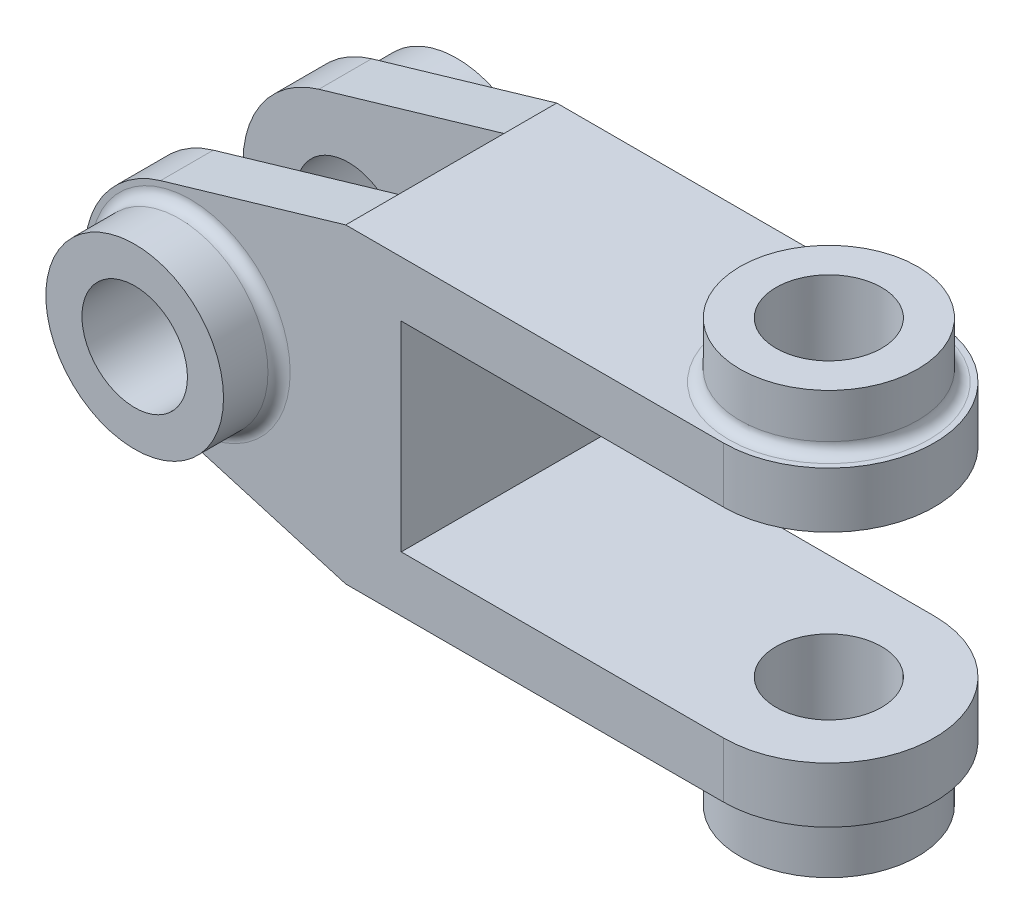
ISO-10303-21;
HEADER;
FILE_DESCRIPTION(('STEP AP214'),'2;1');
FILE_NAME('part.step','',(''),(''),'','','');
FILE_SCHEMA(('AUTOMOTIVE_DESIGN { 1 0 10303 214 1 1 1 1 }'));
ENDSEC;
DATA;
#1=APPLICATION_CONTEXT('core data for automotive mechanical design processes');
#2=APPLICATION_PROTOCOL_DEFINITION('international standard','automotive_design',2000,#1);
#3=PRODUCT_CONTEXT('',#1,'mechanical');
#4=PRODUCT('Part','Part','',(#3));
#5=PRODUCT_RELATED_PRODUCT_CATEGORY('part','',(#4));
#6=PRODUCT_DEFINITION_FORMATION('','',#4);
#7=PRODUCT_DEFINITION_CONTEXT('part definition',#1,'design');
#8=PRODUCT_DEFINITION('design','',#6,#7);
#9=PRODUCT_DEFINITION_SHAPE('','',#8);
#10=(LENGTH_UNIT() NAMED_UNIT(*) SI_UNIT(.MILLI.,.METRE.));
#11=(NAMED_UNIT(*) PLANE_ANGLE_UNIT() SI_UNIT($,.RADIAN.));
#12=(NAMED_UNIT(*) SI_UNIT($,.STERADIAN.) SOLID_ANGLE_UNIT());
#13=UNCERTAINTY_MEASURE_WITH_UNIT(LENGTH_MEASURE(1.E-05),#10,'distance_accuracy_value','');
#14=(GEOMETRIC_REPRESENTATION_CONTEXT(3) GLOBAL_UNCERTAINTY_ASSIGNED_CONTEXT((#13)) GLOBAL_UNIT_ASSIGNED_CONTEXT((#10,
#11,#12)) REPRESENTATION_CONTEXT('',''));
#15=CARTESIAN_POINT('',(0.,0.,0.));
#16=DIRECTION('',(0.,0.,1.));
#17=DIRECTION('',(1.,0.,0.));
#18=AXIS2_PLACEMENT_3D('',#15,#16,#17);
#19=CARTESIAN_POINT('',(0.,0.,19.));
#20=DIRECTION('',(0.,0.,1.));
#21=DIRECTION('',(1.,0.,0.));
#22=AXIS2_PLACEMENT_3D('',#19,#20,#21);
#23=PLANE('',#22);
#24=CARTESIAN_POINT('',(0.,0.,19.));
#25=DIRECTION('',(0.,0.,1.));
#26=DIRECTION('',(1.,0.,0.));
#27=AXIS2_PLACEMENT_3D('',#24,#25,#26);
#28=CIRCLE('',#27,18.);
#29=CARTESIAN_POINT('',(18.,0.,19.));
#30=VERTEX_POINT('',#29);
#31=EDGE_CURVE('E11',#30,#30,#28,.F.);
#32=ORIENTED_EDGE('',*,*,#31,.T.);
#33=EDGE_LOOP('',(#32));
#34=FACE_BOUND('',#33,.T.);
#35=CARTESIAN_POINT('',(0.,0.,19.));
#36=DIRECTION('',(0.,0.,1.));
#37=DIRECTION('',(1.,0.,0.));
#38=AXIS2_PLACEMENT_3D('',#35,#36,#37);
#39=CIRCLE('',#38,19.);
#40=CARTESIAN_POINT('',(-5.34100366267014,18.2338608055273,19.));
#41=VERTEX_POINT('',#40);
#42=CARTESIAN_POINT('',(-5.34100366267014,-18.2338608055273,19.));
#43=VERTEX_POINT('',#42);
#44=EDGE_CURVE('E153',#41,#43,#39,.T.);
#45=ORIENTED_EDGE('',*,*,#44,.T.);
#46=DIRECTION('',(0.959676884501436,-0.281105455930008,0.));
#47=VECTOR('',#46,1.);
#48=CARTESIAN_POINT('',(28.,-28.,19.));
#49=LINE('',#48,#47);
#50=CARTESIAN_POINT('',(28.,-28.,19.));
#51=VERTEX_POINT('',#50);
#52=EDGE_CURVE('E106',#43,#51,#49,.T.);
#53=ORIENTED_EDGE('',*,*,#52,.T.);
#54=DIRECTION('',(1.,0.,0.));
#55=VECTOR('',#54,1.);
#56=CARTESIAN_POINT('',(96.,-28.,19.));
#57=LINE('',#56,#55);
#58=CARTESIAN_POINT('',(96.,-28.,19.));
#59=VERTEX_POINT('',#58);
#60=EDGE_CURVE('E160',#51,#59,#57,.T.);
#61=ORIENTED_EDGE('',*,*,#60,.T.);
#62=DIRECTION('',(0.,1.,0.));
#63=VECTOR('',#62,1.);
#64=CARTESIAN_POINT('',(96.,-18.,19.));
#65=LINE('',#64,#63);
#66=CARTESIAN_POINT('',(96.,-18.,19.));
#67=VERTEX_POINT('',#66);
#68=EDGE_CURVE('E163',#59,#67,#65,.T.);
#69=ORIENTED_EDGE('',*,*,#68,.T.);
#70=DIRECTION('',(-1.,0.,0.));
#71=VECTOR('',#70,1.);
#72=CARTESIAN_POINT('',(38.,-18.,19.));
#73=LINE('',#72,#71);
#74=CARTESIAN_POINT('',(38.,-18.,19.));
#75=VERTEX_POINT('',#74);
#76=EDGE_CURVE('E165',#67,#75,#73,.T.);
#77=ORIENTED_EDGE('',*,*,#76,.T.);
#78=DIRECTION('',(0.,1.,0.));
#79=VECTOR('',#78,1.);
#80=CARTESIAN_POINT('',(38.,18.,19.));
#81=LINE('',#80,#79);
#82=CARTESIAN_POINT('',(38.,18.,19.));
#83=VERTEX_POINT('',#82);
#84=EDGE_CURVE('E168',#75,#83,#81,.T.);
#85=ORIENTED_EDGE('',*,*,#84,.T.);
#86=DIRECTION('',(1.,0.,0.));
#87=VECTOR('',#86,1.);
#88=CARTESIAN_POINT('',(96.,18.,19.));
#89=LINE('',#88,#87);
#90=CARTESIAN_POINT('',(96.,18.,19.));
#91=VERTEX_POINT('',#90);
#92=EDGE_CURVE('E127',#83,#91,#89,.T.);
#93=ORIENTED_EDGE('',*,*,#92,.T.);
#94=DIRECTION('',(0.,1.,0.));
#95=VECTOR('',#94,1.);
#96=CARTESIAN_POINT('',(96.,28.,19.));
#97=LINE('',#96,#95);
#98=CARTESIAN_POINT('',(96.,28.,19.));
#99=VERTEX_POINT('',#98);
#100=EDGE_CURVE('E122',#91,#99,#97,.T.);
#101=ORIENTED_EDGE('',*,*,#100,.T.);
#102=DIRECTION('',(-1.,0.,0.));
#103=VECTOR('',#102,1.);
#104=CARTESIAN_POINT('',(28.,28.,19.));
#105=LINE('',#104,#103);
#106=CARTESIAN_POINT('',(28.,28.,19.));
#107=VERTEX_POINT('',#106);
#108=EDGE_CURVE('E124',#99,#107,#105,.T.);
#109=ORIENTED_EDGE('',*,*,#108,.T.);
#110=DIRECTION('',(-0.959676884501436,-0.281105455930008,0.));
#111=VECTOR('',#110,1.);
#112=CARTESIAN_POINT('',(-5.34100366267014,18.2338608055273,19.));
#113=LINE('',#112,#111);
#114=EDGE_CURVE('E64',#107,#41,#113,.T.);
#115=ORIENTED_EDGE('',*,*,#114,.T.);
#116=EDGE_LOOP('',(#45,#53,#61,#69,#77,#85,#93,#101,#109,#115));
#117=FACE_BOUND('',#116,.T.);
#118=ADVANCED_FACE('F39',(#34,#117),#23,.T.);
#119=CARTESIAN_POINT('',(0.,0.,19.));
#120=DIRECTION('',(0.,0.,-1.));
#121=DIRECTION('',(-1.,0.,0.));
#122=AXIS2_PLACEMENT_3D('',#119,#120,#121);
#123=CYLINDRICAL_SURFACE('',#122,19.);
#124=DIRECTION('',(0.,0.,-1.));
#125=VECTOR('',#124,1.);
#126=CARTESIAN_POINT('',(-5.34100366267014,18.2338608055273,19.));
#127=LINE('',#126,#125);
#128=CARTESIAN_POINT('',(-5.34100366267014,18.2338608055273,9.5));
#129=VERTEX_POINT('',#128);
#130=EDGE_CURVE('E192',#41,#129,#127,.T.);
#131=ORIENTED_EDGE('',*,*,#130,.T.);
#132=CARTESIAN_POINT('',(0.,0.,9.5));
#133=DIRECTION('',(0.,0.,1.));
#134=DIRECTION('',(1.,0.,0.));
#135=AXIS2_PLACEMENT_3D('',#132,#133,#134);
#136=CIRCLE('',#135,19.);
#137=CARTESIAN_POINT('',(-5.34100366267014,-18.2338608055273,9.5));
#138=VERTEX_POINT('',#137);
#139=EDGE_CURVE('E356',#129,#138,#136,.T.);
#140=ORIENTED_EDGE('',*,*,#139,.T.);
#141=DIRECTION('',(0.,0.,-1.));
#142=VECTOR('',#141,1.);
#143=CARTESIAN_POINT('',(-5.34100366267014,-18.2338608055273,19.));
#144=LINE('',#143,#142);
#145=EDGE_CURVE('E206',#43,#138,#144,.T.);
#146=ORIENTED_EDGE('',*,*,#145,.F.);
#147=ORIENTED_EDGE('',*,*,#44,.F.);
#148=EDGE_LOOP('',(#131,#140,#146,#147));
#149=FACE_BOUND('',#148,.T.);
#150=ADVANCED_FACE('F254',(#149),#123,.T.);
#151=CARTESIAN_POINT('',(28.,-28.,19.));
#152=DIRECTION('',(0.281105455930008,0.959676884501436,0.));
#153=DIRECTION('',(-0.959676884501436,0.281105455930008,0.));
#154=AXIS2_PLACEMENT_3D('',#151,#152,#153);
#155=PLANE('',#154);
#156=ORIENTED_EDGE('',*,*,#145,.T.);
#157=DIRECTION('',(0.959676884501436,-0.281105455930008,0.));
#158=VECTOR('',#157,1.);
#159=CARTESIAN_POINT('',(28.,-28.,9.5));
#160=LINE('',#159,#158);
#161=CARTESIAN_POINT('',(28.,-28.,9.5));
#162=VERTEX_POINT('',#161);
#163=EDGE_CURVE('E363',#138,#162,#160,.T.);
#164=ORIENTED_EDGE('',*,*,#163,.T.);
#165=DIRECTION('',(0.,0.,-1.));
#166=VECTOR('',#165,1.);
#167=CARTESIAN_POINT('',(28.,-28.,19.));
#168=LINE('',#167,#166);
#169=EDGE_CURVE('E203',#51,#162,#168,.T.);
#170=ORIENTED_EDGE('',*,*,#169,.F.);
#171=ORIENTED_EDGE('',*,*,#52,.F.);
#172=EDGE_LOOP('',(#156,#164,#170,#171));
#173=FACE_BOUND('',#172,.T.);
#174=ADVANCED_FACE('F264',(#173),#155,.F.);
#175=CARTESIAN_POINT('',(-5.34100366267014,18.2338608055273,19.));
#176=DIRECTION('',(0.281105455930008,-0.959676884501436,0.));
#177=DIRECTION('',(0.959676884501436,0.281105455930008,0.));
#178=AXIS2_PLACEMENT_3D('',#175,#176,#177);
#179=PLANE('',#178);
#180=DIRECTION('',(0.,0.,-1.));
#181=VECTOR('',#180,1.);
#182=CARTESIAN_POINT('',(28.,28.,19.));
#183=LINE('',#182,#181);
#184=CARTESIAN_POINT('',(28.,28.,9.5));
#185=VERTEX_POINT('',#184);
#186=EDGE_CURVE('E138',#107,#185,#183,.T.);
#187=ORIENTED_EDGE('',*,*,#186,.T.);
#188=DIRECTION('',(-0.959676884501436,-0.281105455930008,0.));
#189=VECTOR('',#188,1.);
#190=CARTESIAN_POINT('',(-5.34100366267014,18.2338608055273,9.5));
#191=LINE('',#190,#189);
#192=EDGE_CURVE('E218',#185,#129,#191,.T.);
#193=ORIENTED_EDGE('',*,*,#192,.T.);
#194=ORIENTED_EDGE('',*,*,#130,.F.);
#195=ORIENTED_EDGE('',*,*,#114,.F.);
#196=EDGE_LOOP('',(#187,#193,#194,#195));
#197=FACE_BOUND('',#196,.T.);
#198=ADVANCED_FACE('F280',(#197),#179,.F.);
#199=CARTESIAN_POINT('',(0.,0.,19.));
#200=DIRECTION('',(0.,0.,-1.));
#201=DIRECTION('',(-1.,0.,0.));
#202=AXIS2_PLACEMENT_3D('',#199,#200,#201);
#203=CYLINDRICAL_SURFACE('',#202,9.5);
#204=CARTESIAN_POINT('',(0.,0.,9.5));
#205=DIRECTION('',(0.,0.,1.));
#206=DIRECTION('',(1.,0.,0.));
#207=AXIS2_PLACEMENT_3D('',#204,#205,#206);
#208=CIRCLE('',#207,9.5);
#209=CARTESIAN_POINT('',(9.5,0.,9.5));
#210=VERTEX_POINT('',#209);
#211=EDGE_CURVE('E219',#210,#210,#208,.T.);
#212=ORIENTED_EDGE('',*,*,#211,.F.);
#213=EDGE_LOOP('',(#212));
#214=FACE_BOUND('',#213,.T.);
#215=CARTESIAN_POINT('',(0.,0.,29.));
#216=DIRECTION('',(0.,0.,1.));
#217=DIRECTION('',(1.,0.,0.));
#218=AXIS2_PLACEMENT_3D('',#215,#216,#217);
#219=CIRCLE('',#218,9.5);
#220=CARTESIAN_POINT('',(9.5,0.,29.));
#221=VERTEX_POINT('',#220);
#222=EDGE_CURVE('E336',#221,#221,#219,.T.);
#223=ORIENTED_EDGE('',*,*,#222,.T.);
#224=EDGE_LOOP('',(#223));
#225=FACE_BOUND('',#224,.T.);
#226=ADVANCED_FACE('F272',(#214,#225),#203,.F.);
#227=CARTESIAN_POINT('',(0.,0.,-19.));
#228=DIRECTION('',(0.,0.,1.));
#229=DIRECTION('',(1.,0.,0.));
#230=AXIS2_PLACEMENT_3D('',#227,#228,#229);
#231=PLANE('',#230);
#232=CARTESIAN_POINT('',(0.,0.,-19.));
#233=DIRECTION('',(0.,0.,1.));
#234=DIRECTION('',(1.,0.,0.));
#235=AXIS2_PLACEMENT_3D('',#232,#233,#234);
#236=CIRCLE('',#235,18.);
#237=CARTESIAN_POINT('',(18.,0.,-19.));
#238=VERTEX_POINT('',#237);
#239=EDGE_CURVE('E235',#238,#238,#236,.T.);
#240=ORIENTED_EDGE('',*,*,#239,.T.);
#241=EDGE_LOOP('',(#240));
#242=FACE_BOUND('',#241,.T.);
#243=CARTESIAN_POINT('',(0.,0.,-19.));
#244=DIRECTION('',(0.,0.,1.));
#245=DIRECTION('',(1.,0.,0.));
#246=AXIS2_PLACEMENT_3D('',#243,#244,#245);
#247=CIRCLE('',#246,19.);
#248=CARTESIAN_POINT('',(-5.34100366267014,18.2338608055273,-19.));
#249=VERTEX_POINT('',#248);
#250=CARTESIAN_POINT('',(-5.34100366267014,-18.2338608055273,-19.));
#251=VERTEX_POINT('',#250);
#252=EDGE_CURVE('E149',#249,#251,#247,.T.);
#253=ORIENTED_EDGE('',*,*,#252,.F.);
#254=DIRECTION('',(-0.959676884501436,-0.281105455930008,0.));
#255=VECTOR('',#254,1.);
#256=CARTESIAN_POINT('',(-5.34100366267014,18.2338608055273,-19.));
#257=LINE('',#256,#255);
#258=CARTESIAN_POINT('',(28.,28.,-19.));
#259=VERTEX_POINT('',#258);
#260=EDGE_CURVE('E159',#259,#249,#257,.T.);
#261=ORIENTED_EDGE('',*,*,#260,.F.);
#262=DIRECTION('',(-1.,0.,0.));
#263=VECTOR('',#262,1.);
#264=CARTESIAN_POINT('',(28.,28.,-19.));
#265=LINE('',#264,#263);
#266=CARTESIAN_POINT('',(96.,28.,-19.));
#267=VERTEX_POINT('',#266);
#268=EDGE_CURVE('E189',#267,#259,#265,.T.);
#269=ORIENTED_EDGE('',*,*,#268,.F.);
#270=DIRECTION('',(0.,1.,0.));
#271=VECTOR('',#270,1.);
#272=CARTESIAN_POINT('',(96.,28.,-19.));
#273=LINE('',#272,#271);
#274=CARTESIAN_POINT('',(96.,18.,-19.));
#275=VERTEX_POINT('',#274);
#276=EDGE_CURVE('E144',#275,#267,#273,.T.);
#277=ORIENTED_EDGE('',*,*,#276,.F.);
#278=DIRECTION('',(1.,0.,0.));
#279=VECTOR('',#278,1.);
#280=CARTESIAN_POINT('',(96.,18.,-19.));
#281=LINE('',#280,#279);
#282=CARTESIAN_POINT('',(38.,18.,-19.));
#283=VERTEX_POINT('',#282);
#284=EDGE_CURVE('E183',#283,#275,#281,.T.);
#285=ORIENTED_EDGE('',*,*,#284,.F.);
#286=DIRECTION('',(0.,1.,0.));
#287=VECTOR('',#286,1.);
#288=CARTESIAN_POINT('',(38.,18.,-19.));
#289=LINE('',#288,#287);
#290=CARTESIAN_POINT('',(38.,-18.,-19.));
#291=VERTEX_POINT('',#290);
#292=EDGE_CURVE('E185',#291,#283,#289,.T.);
#293=ORIENTED_EDGE('',*,*,#292,.F.);
#294=DIRECTION('',(-1.,0.,0.));
#295=VECTOR('',#294,1.);
#296=CARTESIAN_POINT('',(38.,-18.,-19.));
#297=LINE('',#296,#295);
#298=CARTESIAN_POINT('',(96.,-18.,-19.));
#299=VERTEX_POINT('',#298);
#300=EDGE_CURVE('E179',#299,#291,#297,.T.);
#301=ORIENTED_EDGE('',*,*,#300,.F.);
#302=DIRECTION('',(0.,1.,0.));
#303=VECTOR('',#302,1.);
#304=CARTESIAN_POINT('',(96.,-18.,-19.));
#305=LINE('',#304,#303);
#306=CARTESIAN_POINT('',(96.,-28.,-19.));
#307=VERTEX_POINT('',#306);
#308=EDGE_CURVE('E180',#307,#299,#305,.T.);
#309=ORIENTED_EDGE('',*,*,#308,.F.);
#310=DIRECTION('',(1.,0.,0.));
#311=VECTOR('',#310,1.);
#312=CARTESIAN_POINT('',(96.,-28.,-19.));
#313=LINE('',#312,#311);
#314=CARTESIAN_POINT('',(28.,-28.,-19.));
#315=VERTEX_POINT('',#314);
#316=EDGE_CURVE('E172',#315,#307,#313,.T.);
#317=ORIENTED_EDGE('',*,*,#316,.F.);
#318=DIRECTION('',(0.959676884501436,-0.281105455930008,0.));
#319=VECTOR('',#318,1.);
#320=CARTESIAN_POINT('',(28.,-28.,-19.));
#321=LINE('',#320,#319);
#322=EDGE_CURVE('E171',#251,#315,#321,.T.);
#323=ORIENTED_EDGE('',*,*,#322,.F.);
#324=EDGE_LOOP('',(#253,#261,#269,#277,#285,#293,#301,#309,#317,#323));
#325=FACE_BOUND('',#324,.T.);
#326=ADVANCED_FACE('F268',(#242,#325),#231,.F.);
#327=CARTESIAN_POINT('',(0.,0.,-9.5));
#328=DIRECTION('',(0.,0.,-1.));
#329=DIRECTION('',(-1.,0.,0.));
#330=AXIS2_PLACEMENT_3D('',#327,#328,#329);
#331=CIRCLE('',#330,19.);
#332=CARTESIAN_POINT('',(-5.34100366267014,-18.2338608055273,-9.5));
#333=VERTEX_POINT('',#332);
#334=CARTESIAN_POINT('',(-5.34100366267014,18.2338608055273,-9.5));
#335=VERTEX_POINT('',#334);
#336=EDGE_CURVE('E351',#333,#335,#331,.T.);
#337=ORIENTED_EDGE('',*,*,#336,.T.);
#338=EDGE_CURVE('E97',#335,#249,#127,.T.);
#339=ORIENTED_EDGE('',*,*,#338,.T.);
#340=ORIENTED_EDGE('',*,*,#252,.T.);
#341=EDGE_CURVE('E210',#333,#251,#144,.T.);
#342=ORIENTED_EDGE('',*,*,#341,.F.);
#343=EDGE_LOOP('',(#337,#339,#340,#342));
#344=FACE_BOUND('',#343,.T.);
#345=ADVANCED_FACE('F263',(#344),#123,.T.);
#346=CARTESIAN_POINT('',(28.,-28.,-9.5));
#347=VERTEX_POINT('',#346);
#348=EDGE_CURVE('E205',#347,#315,#168,.T.);
#349=ORIENTED_EDGE('',*,*,#348,.F.);
#350=DIRECTION('',(-0.959676884501436,0.281105455930008,0.));
#351=VECTOR('',#350,1.);
#352=CARTESIAN_POINT('',(28.,-28.,-9.5));
#353=LINE('',#352,#351);
#354=EDGE_CURVE('E217',#347,#333,#353,.T.);
#355=ORIENTED_EDGE('',*,*,#354,.T.);
#356=ORIENTED_EDGE('',*,*,#341,.T.);
#357=ORIENTED_EDGE('',*,*,#322,.T.);
#358=EDGE_LOOP('',(#349,#355,#356,#357));
#359=FACE_BOUND('',#358,.T.);
#360=ADVANCED_FACE('F298',(#359),#155,.F.);
#361=CARTESIAN_POINT('',(96.,-28.,19.));
#362=DIRECTION('',(0.,1.,0.));
#363=DIRECTION('',(-1.,0.,0.));
#364=AXIS2_PLACEMENT_3D('',#361,#362,#363);
#365=PLANE('',#364);
#366=CARTESIAN_POINT('',(96.,-28.,0.));
#367=DIRECTION('',(0.,1.,0.));
#368=DIRECTION('',(-1.,0.,0.));
#369=AXIS2_PLACEMENT_3D('',#366,#367,#368);
#370=CIRCLE('',#369,18.);
#371=CARTESIAN_POINT('',(78.,-28.,0.));
#372=VERTEX_POINT('',#371);
#373=EDGE_CURVE('E208',#372,#372,#370,.T.);
#374=ORIENTED_EDGE('',*,*,#373,.T.);
#375=EDGE_LOOP('',(#374));
#376=FACE_BOUND('',#375,.T.);
#377=ORIENTED_EDGE('',*,*,#316,.T.);
#378=CARTESIAN_POINT('',(96.,-28.,0.));
#379=DIRECTION('',(0.,-1.,0.));
#380=DIRECTION('',(1.,0.,0.));
#381=AXIS2_PLACEMENT_3D('',#378,#379,#380);
#382=CIRCLE('',#381,19.);
#383=EDGE_CURVE('E148',#307,#59,#382,.T.);
#384=ORIENTED_EDGE('',*,*,#383,.T.);
#385=ORIENTED_EDGE('',*,*,#60,.F.);
#386=ORIENTED_EDGE('',*,*,#169,.T.);
#387=DIRECTION('',(0.,0.,1.));
#388=VECTOR('',#387,1.);
#389=CARTESIAN_POINT('',(28.,-28.,9.5));
#390=LINE('',#389,#388);
#391=EDGE_CURVE('E341',#347,#162,#390,.T.);
#392=ORIENTED_EDGE('',*,*,#391,.F.);
#393=ORIENTED_EDGE('',*,*,#348,.T.);
#394=EDGE_LOOP('',(#377,#384,#385,#386,#392,#393));
#395=FACE_BOUND('',#394,.T.);
#396=ADVANCED_FACE('F292',(#376,#395),#365,.F.);
#397=CARTESIAN_POINT('',(38.,-18.,19.));
#398=DIRECTION('',(0.,-1.,0.));
#399=DIRECTION('',(1.,0.,0.));
#400=AXIS2_PLACEMENT_3D('',#397,#398,#399);
#401=PLANE('',#400);
#402=CARTESIAN_POINT('',(96.,-18.,0.));
#403=DIRECTION('',(0.,-1.,0.));
#404=DIRECTION('',(1.,0.,0.));
#405=AXIS2_PLACEMENT_3D('',#402,#403,#404);
#406=CIRCLE('',#405,9.49999999999999);
#407=CARTESIAN_POINT('',(105.5,-18.,0.));
#408=VERTEX_POINT('',#407);
#409=EDGE_CURVE('E331',#408,#408,#406,.T.);
#410=ORIENTED_EDGE('',*,*,#409,.T.);
#411=EDGE_LOOP('',(#410));
#412=FACE_BOUND('',#411,.T.);
#413=ORIENTED_EDGE('',*,*,#76,.F.);
#414=CARTESIAN_POINT('',(96.,-18.,0.));
#415=DIRECTION('',(0.,-1.,0.));
#416=DIRECTION('',(1.,0.,0.));
#417=AXIS2_PLACEMENT_3D('',#414,#415,#416);
#418=CIRCLE('',#417,19.);
#419=EDGE_CURVE('E147',#67,#299,#418,.F.);
#420=ORIENTED_EDGE('',*,*,#419,.T.);
#421=ORIENTED_EDGE('',*,*,#300,.T.);
#422=DIRECTION('',(0.,0.,-1.));
#423=VECTOR('',#422,1.);
#424=CARTESIAN_POINT('',(38.,-18.,19.));
#425=LINE('',#424,#423);
#426=EDGE_CURVE('E197',#75,#291,#425,.T.);
#427=ORIENTED_EDGE('',*,*,#426,.F.);
#428=EDGE_LOOP('',(#413,#420,#421,#427));
#429=FACE_BOUND('',#428,.T.);
#430=ADVANCED_FACE('F290',(#412,#429),#401,.F.);
#431=CARTESIAN_POINT('',(38.,18.,19.));
#432=DIRECTION('',(-1.,0.,0.));
#433=DIRECTION('',(0.,0.,1.));
#434=AXIS2_PLACEMENT_3D('',#431,#432,#433);
#435=PLANE('',#434);
#436=ORIENTED_EDGE('',*,*,#292,.T.);
#437=DIRECTION('',(0.,0.,-1.));
#438=VECTOR('',#437,1.);
#439=CARTESIAN_POINT('',(38.,18.,19.));
#440=LINE('',#439,#438);
#441=EDGE_CURVE('E199',#83,#283,#440,.T.);
#442=ORIENTED_EDGE('',*,*,#441,.F.);
#443=ORIENTED_EDGE('',*,*,#84,.F.);
#444=ORIENTED_EDGE('',*,*,#426,.T.);
#445=EDGE_LOOP('',(#436,#442,#443,#444));
#446=FACE_BOUND('',#445,.T.);
#447=ADVANCED_FACE('F283',(#446),#435,.F.);
#448=CARTESIAN_POINT('',(96.,18.,19.));
#449=DIRECTION('',(0.,1.,0.));
#450=DIRECTION('',(-1.,0.,0.));
#451=AXIS2_PLACEMENT_3D('',#448,#449,#450);
#452=PLANE('',#451);
#453=CARTESIAN_POINT('',(96.,18.,0.));
#454=DIRECTION('',(0.,1.,0.));
#455=DIRECTION('',(-1.,0.,0.));
#456=AXIS2_PLACEMENT_3D('',#453,#454,#455);
#457=CIRCLE('',#456,9.49999999999999);
#458=CARTESIAN_POINT('',(86.5,18.,0.));
#459=VERTEX_POINT('',#458);
#460=EDGE_CURVE('E470',#459,#459,#457,.T.);
#461=ORIENTED_EDGE('',*,*,#460,.T.);
#462=EDGE_LOOP('',(#461));
#463=FACE_BOUND('',#462,.T.);
#464=ORIENTED_EDGE('',*,*,#284,.T.);
#465=CARTESIAN_POINT('',(96.,18.,0.));
#466=DIRECTION('',(0.,1.,0.));
#467=DIRECTION('',(-1.,0.,0.));
#468=AXIS2_PLACEMENT_3D('',#465,#466,#467);
#469=CIRCLE('',#468,19.);
#470=EDGE_CURVE('E143',#275,#91,#469,.F.);
#471=ORIENTED_EDGE('',*,*,#470,.T.);
#472=ORIENTED_EDGE('',*,*,#92,.F.);
#473=ORIENTED_EDGE('',*,*,#441,.T.);
#474=EDGE_LOOP('',(#464,#471,#472,#473));
#475=FACE_BOUND('',#474,.T.);
#476=ADVANCED_FACE('F278',(#463,#475),#452,.F.);
#477=CARTESIAN_POINT('',(28.,28.,19.));
#478=DIRECTION('',(0.,-1.,0.));
#479=DIRECTION('',(1.,0.,0.));
#480=AXIS2_PLACEMENT_3D('',#477,#478,#479);
#481=PLANE('',#480);
#482=CARTESIAN_POINT('',(96.,28.,0.));
#483=DIRECTION('',(0.,-1.,0.));
#484=DIRECTION('',(1.,0.,0.));
#485=AXIS2_PLACEMENT_3D('',#482,#483,#484);
#486=CIRCLE('',#485,18.);
#487=CARTESIAN_POINT('',(114.,28.,0.));
#488=VERTEX_POINT('',#487);
#489=EDGE_CURVE('E230',#488,#488,#486,.T.);
#490=ORIENTED_EDGE('',*,*,#489,.T.);
#491=EDGE_LOOP('',(#490));
#492=FACE_BOUND('',#491,.T.);
#493=ORIENTED_EDGE('',*,*,#108,.F.);
#494=CARTESIAN_POINT('',(96.,28.,0.));
#495=DIRECTION('',(0.,1.,0.));
#496=DIRECTION('',(-1.,0.,0.));
#497=AXIS2_PLACEMENT_3D('',#494,#495,#496);
#498=CIRCLE('',#497,19.);
#499=EDGE_CURVE('E139',#99,#267,#498,.T.);
#500=ORIENTED_EDGE('',*,*,#499,.T.);
#501=ORIENTED_EDGE('',*,*,#268,.T.);
#502=CARTESIAN_POINT('',(28.,28.,-9.5));
#503=VERTEX_POINT('',#502);
#504=EDGE_CURVE('E191',#503,#259,#183,.T.);
#505=ORIENTED_EDGE('',*,*,#504,.F.);
#506=EDGE_CURVE('E196',#185,#503,#183,.T.);
#507=ORIENTED_EDGE('',*,*,#506,.F.);
#508=ORIENTED_EDGE('',*,*,#186,.F.);
#509=EDGE_LOOP('',(#493,#500,#501,#505,#507,#508));
#510=FACE_BOUND('',#509,.T.);
#511=ADVANCED_FACE('F133',(#492,#510),#481,.F.);
#512=ORIENTED_EDGE('',*,*,#338,.F.);
#513=DIRECTION('',(0.959676884501436,0.281105455930008,0.));
#514=VECTOR('',#513,1.);
#515=CARTESIAN_POINT('',(-5.34100366267014,18.2338608055273,-9.5));
#516=LINE('',#515,#514);
#517=EDGE_CURVE('E211',#335,#503,#516,.T.);
#518=ORIENTED_EDGE('',*,*,#517,.T.);
#519=ORIENTED_EDGE('',*,*,#504,.T.);
#520=ORIENTED_EDGE('',*,*,#260,.T.);
#521=EDGE_LOOP('',(#512,#518,#519,#520));
#522=FACE_BOUND('',#521,.T.);
#523=ADVANCED_FACE('F271',(#522),#179,.F.);
#524=CARTESIAN_POINT('',(0.,0.,-9.5));
#525=DIRECTION('',(0.,0.,-1.));
#526=DIRECTION('',(-1.,0.,0.));
#527=AXIS2_PLACEMENT_3D('',#524,#525,#526);
#528=CIRCLE('',#527,9.5);
#529=CARTESIAN_POINT('',(-9.5,0.,-9.5));
#530=VERTEX_POINT('',#529);
#531=EDGE_CURVE('E212',#530,#530,#528,.T.);
#532=ORIENTED_EDGE('',*,*,#531,.F.);
#533=EDGE_LOOP('',(#532));
#534=FACE_BOUND('',#533,.T.);
#535=CARTESIAN_POINT('',(0.,0.,-29.));
#536=DIRECTION('',(0.,0.,1.));
#537=DIRECTION('',(1.,0.,0.));
#538=AXIS2_PLACEMENT_3D('',#535,#536,#537);
#539=CIRCLE('',#538,9.5);
#540=CARTESIAN_POINT('',(9.5,0.,-29.));
#541=VERTEX_POINT('',#540);
#542=EDGE_CURVE('E323',#541,#541,#539,.T.);
#543=ORIENTED_EDGE('',*,*,#542,.F.);
#544=EDGE_LOOP('',(#543));
#545=FACE_BOUND('',#544,.T.);
#546=ADVANCED_FACE('F266',(#534,#545),#203,.F.);
#547=CARTESIAN_POINT('',(96.,-35.7401153701776,0.));
#548=DIRECTION('',(0.,1.,0.));
#549=DIRECTION('',(-1.,0.,0.));
#550=AXIS2_PLACEMENT_3D('',#547,#548,#549);
#551=CYLINDRICAL_SURFACE('',#550,19.);
#552=ORIENTED_EDGE('',*,*,#100,.F.);
#553=ORIENTED_EDGE('',*,*,#470,.F.);
#554=ORIENTED_EDGE('',*,*,#276,.T.);
#555=ORIENTED_EDGE('',*,*,#499,.F.);
#556=EDGE_LOOP('',(#552,#553,#554,#555));
#557=FACE_BOUND('',#556,.T.);
#558=ADVANCED_FACE('F145',(#557),#551,.T.);
#559=CARTESIAN_POINT('',(96.,35.7401153701776,0.));
#560=DIRECTION('',(0.,-1.,0.));
#561=DIRECTION('',(1.,0.,0.));
#562=AXIS2_PLACEMENT_3D('',#559,#560,#561);
#563=CYLINDRICAL_SURFACE('',#562,19.);
#564=ORIENTED_EDGE('',*,*,#308,.T.);
#565=ORIENTED_EDGE('',*,*,#419,.F.);
#566=ORIENTED_EDGE('',*,*,#68,.F.);
#567=ORIENTED_EDGE('',*,*,#383,.F.);
#568=EDGE_LOOP('',(#564,#565,#566,#567));
#569=FACE_BOUND('',#568,.T.);
#570=ADVANCED_FACE('F411',(#569),#563,.T.);
#571=CARTESIAN_POINT('',(28.,39.,9.5));
#572=DIRECTION('',(1.,0.,0.));
#573=DIRECTION('',(0.,1.,0.));
#574=AXIS2_PLACEMENT_3D('',#571,#572,#573);
#575=PLANE('',#574);
#576=DIRECTION('',(0.,-1.,0.));
#577=VECTOR('',#576,1.);
#578=CARTESIAN_POINT('',(28.,39.,-9.5));
#579=LINE('',#578,#577);
#580=EDGE_CURVE('E53',#503,#347,#579,.T.);
#581=ORIENTED_EDGE('',*,*,#580,.T.);
#582=ORIENTED_EDGE('',*,*,#391,.T.);
#583=DIRECTION('',(0.,-1.,0.));
#584=VECTOR('',#583,1.);
#585=CARTESIAN_POINT('',(28.,39.,9.5));
#586=LINE('',#585,#584);
#587=EDGE_CURVE('E213',#185,#162,#586,.T.);
#588=ORIENTED_EDGE('',*,*,#587,.F.);
#589=ORIENTED_EDGE('',*,*,#506,.T.);
#590=EDGE_LOOP('',(#581,#582,#588,#589));
#591=FACE_BOUND('',#590,.T.);
#592=ADVANCED_FACE('F413',(#591),#575,.F.);
#593=CARTESIAN_POINT('',(-19.,39.,9.5));
#594=DIRECTION('',(0.,0.,1.));
#595=DIRECTION('',(1.,0.,0.));
#596=AXIS2_PLACEMENT_3D('',#593,#594,#595);
#597=PLANE('',#596);
#598=ORIENTED_EDGE('',*,*,#211,.T.);
#599=EDGE_LOOP('',(#598));
#600=FACE_BOUND('',#599,.T.);
#601=ORIENTED_EDGE('',*,*,#139,.F.);
#602=ORIENTED_EDGE('',*,*,#192,.F.);
#603=ORIENTED_EDGE('',*,*,#587,.T.);
#604=ORIENTED_EDGE('',*,*,#163,.F.);
#605=EDGE_LOOP('',(#601,#602,#603,#604));
#606=FACE_BOUND('',#605,.T.);
#607=ADVANCED_FACE('F417',(#600,#606),#597,.F.);
#608=CARTESIAN_POINT('',(-19.,39.,-9.5));
#609=DIRECTION('',(0.,0.,-1.));
#610=DIRECTION('',(-1.,0.,0.));
#611=AXIS2_PLACEMENT_3D('',#608,#609,#610);
#612=PLANE('',#611);
#613=ORIENTED_EDGE('',*,*,#531,.T.);
#614=EDGE_LOOP('',(#613));
#615=FACE_BOUND('',#614,.T.);
#616=ORIENTED_EDGE('',*,*,#580,.F.);
#617=ORIENTED_EDGE('',*,*,#517,.F.);
#618=ORIENTED_EDGE('',*,*,#336,.F.);
#619=ORIENTED_EDGE('',*,*,#354,.F.);
#620=EDGE_LOOP('',(#616,#617,#618,#619));
#621=FACE_BOUND('',#620,.T.);
#622=ADVANCED_FACE('F425',(#615,#621),#612,.F.);
#623=CARTESIAN_POINT('',(0.,0.,29.));
#624=DIRECTION('',(0.,0.,1.));
#625=DIRECTION('',(1.,0.,0.));
#626=AXIS2_PLACEMENT_3D('',#623,#624,#625);
#627=PLANE('',#626);
#628=CARTESIAN_POINT('',(0.,0.,29.));
#629=DIRECTION('',(0.,0.,1.));
#630=DIRECTION('',(1.,0.,0.));
#631=AXIS2_PLACEMENT_3D('',#628,#629,#630);
#632=CIRCLE('',#631,16.);
#633=CARTESIAN_POINT('',(16.,0.,29.));
#634=VERTEX_POINT('',#633);
#635=EDGE_CURVE('E342',#634,#634,#632,.T.);
#636=ORIENTED_EDGE('',*,*,#635,.T.);
#637=EDGE_LOOP('',(#636));
#638=FACE_BOUND('',#637,.T.);
#639=ORIENTED_EDGE('',*,*,#222,.F.);
#640=EDGE_LOOP('',(#639));
#641=FACE_BOUND('',#640,.T.);
#642=ADVANCED_FACE('F428',(#638,#641),#627,.T.);
#643=CARTESIAN_POINT('',(0.,0.,29.));
#644=DIRECTION('',(0.,0.,-1.));
#645=DIRECTION('',(-1.,0.,0.));
#646=AXIS2_PLACEMENT_3D('',#643,#644,#645);
#647=CYLINDRICAL_SURFACE('',#646,16.);
#648=CARTESIAN_POINT('',(0.,0.,21.));
#649=DIRECTION('',(0.,0.,1.));
#650=DIRECTION('',(1.,0.,0.));
#651=AXIS2_PLACEMENT_3D('',#648,#649,#650);
#652=CIRCLE('',#651,16.);
#653=CARTESIAN_POINT('',(16.,0.,21.));
#654=VERTEX_POINT('',#653);
#655=EDGE_CURVE('E50',#654,#654,#652,.T.);
#656=ORIENTED_EDGE('',*,*,#655,.T.);
#657=EDGE_LOOP('',(#656));
#658=FACE_BOUND('',#657,.T.);
#659=ORIENTED_EDGE('',*,*,#635,.F.);
#660=EDGE_LOOP('',(#659));
#661=FACE_BOUND('',#660,.T.);
#662=ADVANCED_FACE('F239',(#658,#661),#647,.T.);
#663=CARTESIAN_POINT('',(0.,0.,-29.));
#664=DIRECTION('',(0.,0.,1.));
#665=DIRECTION('',(1.,0.,0.));
#666=AXIS2_PLACEMENT_3D('',#663,#664,#665);
#667=CYLINDRICAL_SURFACE('',#666,16.);
#668=CARTESIAN_POINT('',(0.,0.,-21.));
#669=DIRECTION('',(0.,0.,1.));
#670=DIRECTION('',(1.,0.,0.));
#671=AXIS2_PLACEMENT_3D('',#668,#669,#670);
#672=CIRCLE('',#671,16.);
#673=CARTESIAN_POINT('',(16.,0.,-21.));
#674=VERTEX_POINT('',#673);
#675=EDGE_CURVE('E232',#674,#674,#672,.F.);
#676=ORIENTED_EDGE('',*,*,#675,.T.);
#677=EDGE_LOOP('',(#676));
#678=FACE_BOUND('',#677,.T.);
#679=CARTESIAN_POINT('',(0.,0.,-29.));
#680=DIRECTION('',(0.,0.,1.));
#681=DIRECTION('',(1.,0.,0.));
#682=AXIS2_PLACEMENT_3D('',#679,#680,#681);
#683=CIRCLE('',#682,16.);
#684=CARTESIAN_POINT('',(16.,0.,-29.));
#685=VERTEX_POINT('',#684);
#686=EDGE_CURVE('E328',#685,#685,#683,.T.);
#687=ORIENTED_EDGE('',*,*,#686,.T.);
#688=EDGE_LOOP('',(#687));
#689=FACE_BOUND('',#688,.T.);
#690=ADVANCED_FACE('F432',(#678,#689),#667,.T.);
#691=CARTESIAN_POINT('',(0.,0.,-29.));
#692=DIRECTION('',(0.,0.,-1.));
#693=DIRECTION('',(1.,0.,0.));
#694=AXIS2_PLACEMENT_3D('',#691,#692,#693);
#695=PLANE('',#694);
#696=ORIENTED_EDGE('',*,*,#542,.T.);
#697=EDGE_LOOP('',(#696));
#698=FACE_BOUND('',#697,.T.);
#699=ORIENTED_EDGE('',*,*,#686,.F.);
#700=EDGE_LOOP('',(#699));
#701=FACE_BOUND('',#700,.T.);
#702=ADVANCED_FACE('F316',(#698,#701),#695,.T.);
#703=CARTESIAN_POINT('',(96.,38.,0.));
#704=DIRECTION('',(0.,-1.,0.));
#705=DIRECTION('',(1.,0.,0.));
#706=AXIS2_PLACEMENT_3D('',#703,#704,#705);
#707=CYLINDRICAL_SURFACE('',#706,16.);
#708=CARTESIAN_POINT('',(96.,30.,0.));
#709=DIRECTION('',(0.,-1.,0.));
#710=DIRECTION('',(1.,0.,0.));
#711=AXIS2_PLACEMENT_3D('',#708,#709,#710);
#712=CIRCLE('',#711,16.);
#713=CARTESIAN_POINT('',(112.,30.,0.));
#714=VERTEX_POINT('',#713);
#715=EDGE_CURVE('E228',#714,#714,#712,.F.);
#716=ORIENTED_EDGE('',*,*,#715,.T.);
#717=EDGE_LOOP('',(#716));
#718=FACE_BOUND('',#717,.T.);
#719=CARTESIAN_POINT('',(96.,38.,0.));
#720=DIRECTION('',(0.,1.,0.));
#721=DIRECTION('',(-1.,0.,0.));
#722=AXIS2_PLACEMENT_3D('',#719,#720,#721);
#723=CIRCLE('',#722,16.);
#724=CARTESIAN_POINT('',(80.,38.,0.));
#725=VERTEX_POINT('',#724);
#726=EDGE_CURVE('E324',#725,#725,#723,.T.);
#727=ORIENTED_EDGE('',*,*,#726,.F.);
#728=EDGE_LOOP('',(#727));
#729=FACE_BOUND('',#728,.T.);
#730=ADVANCED_FACE('F314',(#718,#729),#707,.T.);
#731=CARTESIAN_POINT('',(96.,38.,0.));
#732=DIRECTION('',(0.,1.,0.));
#733=DIRECTION('',(-1.,0.,0.));
#734=AXIS2_PLACEMENT_3D('',#731,#732,#733);
#735=PLANE('',#734);
#736=CARTESIAN_POINT('',(96.,38.,0.));
#737=DIRECTION('',(0.,-1.,0.));
#738=DIRECTION('',(1.,0.,0.));
#739=AXIS2_PLACEMENT_3D('',#736,#737,#738);
#740=CIRCLE('',#739,9.49999999999999);
#741=CARTESIAN_POINT('',(105.5,38.,0.));
#742=VERTEX_POINT('',#741);
#743=EDGE_CURVE('E469',#742,#742,#740,.T.);
#744=ORIENTED_EDGE('',*,*,#743,.T.);
#745=EDGE_LOOP('',(#744));
#746=FACE_BOUND('',#745,.T.);
#747=ORIENTED_EDGE('',*,*,#726,.T.);
#748=EDGE_LOOP('',(#747));
#749=FACE_BOUND('',#748,.T.);
#750=ADVANCED_FACE('F319',(#746,#749),#735,.T.);
#751=CARTESIAN_POINT('',(96.,-38.,0.));
#752=DIRECTION('',(0.,1.,0.));
#753=DIRECTION('',(-1.,0.,0.));
#754=AXIS2_PLACEMENT_3D('',#751,#752,#753);
#755=CYLINDRICAL_SURFACE('',#754,16.);
#756=CARTESIAN_POINT('',(96.,-30.,0.));
#757=DIRECTION('',(0.,1.,0.));
#758=DIRECTION('',(-1.,0.,0.));
#759=AXIS2_PLACEMENT_3D('',#756,#757,#758);
#760=CIRCLE('',#759,16.);
#761=CARTESIAN_POINT('',(80.,-30.,0.));
#762=VERTEX_POINT('',#761);
#763=EDGE_CURVE('E225',#762,#762,#760,.F.);
#764=ORIENTED_EDGE('',*,*,#763,.T.);
#765=EDGE_LOOP('',(#764));
#766=FACE_BOUND('',#765,.T.);
#767=CARTESIAN_POINT('',(96.,-38.,0.));
#768=DIRECTION('',(0.,1.,0.));
#769=DIRECTION('',(-1.,0.,0.));
#770=AXIS2_PLACEMENT_3D('',#767,#768,#769);
#771=CIRCLE('',#770,16.);
#772=CARTESIAN_POINT('',(80.,-38.,0.));
#773=VERTEX_POINT('',#772);
#774=EDGE_CURVE('E329',#773,#773,#771,.T.);
#775=ORIENTED_EDGE('',*,*,#774,.T.);
#776=EDGE_LOOP('',(#775));
#777=FACE_BOUND('',#776,.T.);
#778=ADVANCED_FACE('F447',(#766,#777),#755,.T.);
#779=CARTESIAN_POINT('',(96.,-38.,0.));
#780=DIRECTION('',(0.,-1.,0.));
#781=DIRECTION('',(-1.,0.,0.));
#782=AXIS2_PLACEMENT_3D('',#779,#780,#781);
#783=PLANE('',#782);
#784=CARTESIAN_POINT('',(96.,-38.,0.));
#785=DIRECTION('',(0.,-1.,0.));
#786=DIRECTION('',(1.,0.,0.));
#787=AXIS2_PLACEMENT_3D('',#784,#785,#786);
#788=CIRCLE('',#787,9.49999999999999);
#789=CARTESIAN_POINT('',(105.5,-38.,0.));
#790=VERTEX_POINT('',#789);
#791=EDGE_CURVE('E463',#790,#790,#788,.T.);
#792=ORIENTED_EDGE('',*,*,#791,.F.);
#793=EDGE_LOOP('',(#792));
#794=FACE_BOUND('',#793,.T.);
#795=ORIENTED_EDGE('',*,*,#774,.F.);
#796=EDGE_LOOP('',(#795));
#797=FACE_BOUND('',#796,.T.);
#798=ADVANCED_FACE('F448',(#794,#797),#783,.T.);
#799=CARTESIAN_POINT('',(96.,38.,0.));
#800=DIRECTION('',(0.,-1.,0.));
#801=DIRECTION('',(1.,0.,0.));
#802=AXIS2_PLACEMENT_3D('',#799,#800,#801);
#803=CYLINDRICAL_SURFACE('',#802,9.49999999999999);
#804=ORIENTED_EDGE('',*,*,#791,.T.);
#805=EDGE_LOOP('',(#804));
#806=FACE_BOUND('',#805,.T.);
#807=ORIENTED_EDGE('',*,*,#409,.F.);
#808=EDGE_LOOP('',(#807));
#809=FACE_BOUND('',#808,.T.);
#810=ADVANCED_FACE('F451',(#806,#809),#803,.F.);
#811=ORIENTED_EDGE('',*,*,#743,.F.);
#812=EDGE_LOOP('',(#811));
#813=FACE_BOUND('',#812,.T.);
#814=ORIENTED_EDGE('',*,*,#460,.F.);
#815=EDGE_LOOP('',(#814));
#816=FACE_BOUND('',#815,.T.);
#817=ADVANCED_FACE('F304',(#813,#816),#803,.F.);
#818=CARTESIAN_POINT('',(96.,-30.,0.));
#819=DIRECTION('',(0.,1.,0.));
#820=DIRECTION('',(-1.,0.,0.));
#821=AXIS2_PLACEMENT_3D('',#818,#819,#820);
#822=TOROIDAL_SURFACE('',#821,18.,2.);
#823=ORIENTED_EDGE('',*,*,#763,.F.);
#824=EDGE_LOOP('',(#823));
#825=FACE_BOUND('',#824,.T.);
#826=ORIENTED_EDGE('',*,*,#373,.F.);
#827=EDGE_LOOP('',(#826));
#828=FACE_BOUND('',#827,.T.);
#829=ADVANCED_FACE('F305',(#825,#828),#822,.F.);
#830=CARTESIAN_POINT('',(96.,30.,0.));
#831=DIRECTION('',(0.,-1.,0.));
#832=DIRECTION('',(1.,0.,0.));
#833=AXIS2_PLACEMENT_3D('',#830,#831,#832);
#834=TOROIDAL_SURFACE('',#833,18.,2.);
#835=ORIENTED_EDGE('',*,*,#489,.F.);
#836=EDGE_LOOP('',(#835));
#837=FACE_BOUND('',#836,.T.);
#838=ORIENTED_EDGE('',*,*,#715,.F.);
#839=EDGE_LOOP('',(#838));
#840=FACE_BOUND('',#839,.T.);
#841=ADVANCED_FACE('F248',(#837,#840),#834,.F.);
#842=CARTESIAN_POINT('',(0.,0.,-21.));
#843=DIRECTION('',(0.,0.,1.));
#844=DIRECTION('',(1.,0.,0.));
#845=AXIS2_PLACEMENT_3D('',#842,#843,#844);
#846=TOROIDAL_SURFACE('',#845,18.,2.);
#847=ORIENTED_EDGE('',*,*,#675,.F.);
#848=EDGE_LOOP('',(#847));
#849=FACE_BOUND('',#848,.T.);
#850=ORIENTED_EDGE('',*,*,#239,.F.);
#851=EDGE_LOOP('',(#850));
#852=FACE_BOUND('',#851,.T.);
#853=ADVANCED_FACE('F242',(#849,#852),#846,.F.);
#854=CARTESIAN_POINT('',(0.,0.,21.));
#855=DIRECTION('',(0.,0.,1.));
#856=DIRECTION('',(1.,0.,0.));
#857=AXIS2_PLACEMENT_3D('',#854,#855,#856);
#858=TOROIDAL_SURFACE('',#857,18.,2.);
#859=ORIENTED_EDGE('',*,*,#31,.F.);
#860=EDGE_LOOP('',(#859));
#861=FACE_BOUND('',#860,.T.);
#862=ORIENTED_EDGE('',*,*,#655,.F.);
#863=EDGE_LOOP('',(#862));
#864=FACE_BOUND('',#863,.T.);
#865=ADVANCED_FACE('F41',(#861,#864),#858,.F.);
#866=CLOSED_SHELL('',(#118,#150,#174,#198,#226,#326,#345,#360,#396,#430,#447,#476,#511,#523,
#546,#558,#570,#592,#607,#622,#642,#662,#690,#702,#730,#750,#778,#798,#810,#817,#829,#841,#853,#865));
#867=MANIFOLD_SOLID_BREP('B2',#866);
#868=ADVANCED_BREP_SHAPE_REPRESENTATION('',(#18,#867),#14);
#869=SHAPE_DEFINITION_REPRESENTATION(#9,#868);
ENDSEC;
END-ISO-10303-21;
